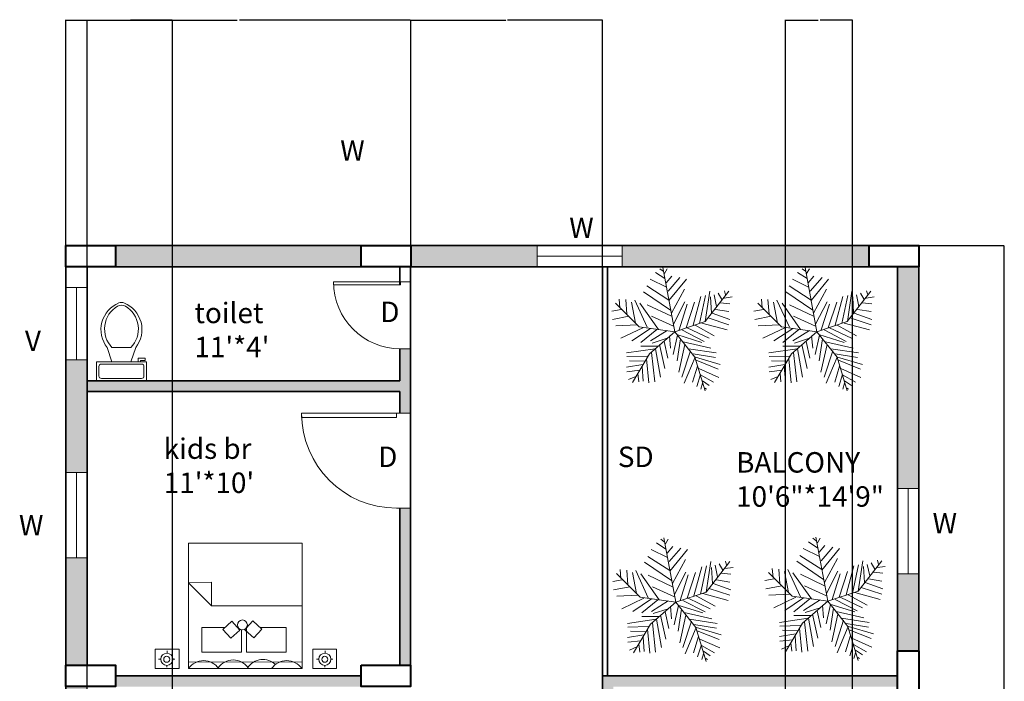
# Model space of a CAD drawing. Units: inches. Extents: x 1568 to 2529, y 2149 to 2897.
# Tile 16 of 16: x 2113 to 2529, y 2618 to 2897. Entities that reach past the tile are written whole.
import ezdxf

# ---------------------------------------------------------------- set-up
doc = ezdxf.new("R2010")
doc.units = ezdxf.units.IN
for name, color, linetype, lineweight in [('A-ANNO-DIMS', 2, 'Continuous', 18), ('A-AREA-IDEN', 210, 'Continuous', 18), ('A-COLS', 7, 'Continuous', 40), ('A-DOOR', 4, 'Continuous', 18), ('A-FLOR-FIXT', 9, 'Continuous', 18), ('A-FURN', 8, 'Continuous', 18), ('A-WALL-PATT', 172, 'Continuous', 13), ('text', 210, 'Continuous', 18), ('TREE', 94, 'Continuous', 13), ('wall', 7, 'Continuous', 35), ('window', 130, 'Continuous', 18)]:
    doc.layers.add(name, color=color, linetype=linetype, lineweight=lineweight)
doc.styles.get("Standard").update_dxf_attribs({"font": 'arial.ttf'})
doc.dimstyles.get("Standard").update_dxf_attribs({"dimtxt": 0.18, "dimasz": 0.18, "dimexe": 0.18, "dimexo": 0.0625, "dimgap": 0.09, "dimtad": 0, "dimtih": 1, "dimtoh": 1, "dimdec": 4, "dimzin": 0, "dimdsep": 46, "dimtxsty": 'Standard', "dimcen": 0.09, "dimadec": 0, "dimazin": 0, "dimtfac": 1, "dimtdec": 4, "dimtofl": 0, "dimtmove": 0, "dimatfit": 3, "dimfxl": 1, "dimtolj": 1, "dimtzin": 0, "dimarcsym": 0})

# ---------------------------------------------------------------- blocks, each defined once
blk = doc.blocks.new('*U4')
for p, q in [((9.5, -6), (9.5, -2)), ((-8, -8.5), (-8, -8)), ((-7, -8), (-7, -9.5)), ((-4, -8), (-6, -14)), ((4, -8), (6, -14)), ((-10, -8.5), (-8, -8.5)), ((-10, -9.5), (-10, -8.5)), ((-7, -9.5), (-10, -9.5)), ((4, -14), (-4, -14))]:
    blk.add_line(p, q)
blk.add_lwpolyline([(10.5, -8), (10.5, 0), (-10.5, 0), (-10.5, -8)], close=True)
for points in [[(-9.5, -2), (-9.5, -6)], [(8.5, -1), (-8.5, -1)], [(-8.5, -7), (8.5, -7)]]:
    blk.add_lwpolyline(points)
for centre, radius, start, end in [((-8.62, -1.88), 0.884, 81.8699, 188.1301), ((8.62, -1.88), 0.884, 351.8699, 98.1301), ((-8.62, -6.12), 0.884, 171.8699, 278.1301), ((8.62, -6.12), 0.884, 261.8699, 8.1301), ((3.52, -21.58), 12.17, 141.4691, 247.9714), ((4.2, -21.82), 11.33, 136.3677, 238.9468), ((-3.52, -21.58), 12.17, 292.0284, 38.5307), ((-4.2, -21.82), 11.33, 301.053, 43.6321), ((0, -27.88), 4, 245.7318, 294.2682), ((0, -29), 4, 254.8605, 285.1395)]:
    blk.add_arc(centre, radius, start, end)
blk = doc.blocks.new('*U2')
for p, q in [((0, 0), (0, -6)), ((40, 0), (40, -6))]:
    blk.add_line(p, q)
blk.add_lwpolyline([(0, 0), (0, 40), (1.75, 40), (1.75, 0)], close=True)
blk.add_arc((0, 0), 40, 0, 90)
blk = doc.blocks.new('*U10')
for p, q in [((-8.737, 47.138), (-17.069, 52.711)), ((-10.186, 53.64), (-13.084, 55.962)), ((0, 0), (-10.5, 57)), ((-9.099, 51.782), (-6.563, 55.962)), ((-7.288, 39.707), (-21.778, 46.673)), ((-7.65, 43.423), (-2.578, 49.46)), ((-5.839, 35.992), (4.667, 48.067)), ((-5.114, 27.632), (10.463, 46.673)), ((-3.665, 19.273), (-27.574, 35.527)), ((-5.114, 28.097), (-24.676, 40.636)), ((-2.941, 16.486), (8.652, 37.85)), ((27, 9), (48, 36)), ((27.127, 9.056), (31.112, 35.992)), ((44.153, 36.456), (45.239, 32.741)), ((-48.585, 21.131), (-49.309, 29.026)), ((-43.513, 28.561), (-42.427, 15.558)), ((-38.442, 26.239), (-34.819, 7.663)), ((-35.544, 28.097), (-24.314, 3.947)), ((-1.129, 6.734), (9.014, 26.704)), ((10.101, 3.483), (17.708, 26.239)), ((16.259, 5.805), (23.142, 31.348)), ((22.055, 7.198), (27.489, 32.277)), ((31.836, 30.883), (32.561, 16.486)), ((35.096, 32.741), (37.27, 22.524)), ((38.719, 34.134), (41.979, 28.561)), ((43.791, 29.954), (51.036, 30.883)), ((-47.498, 19.737), (-55.83, 18.344)), ((-31.5, 4.5), (-52.5, 25.5)), ((-14.533, 2.09), (-30.834, 25.31)), ((-24.314, 23.917), (-2.941, 13.7)), ((3.942, 1.625), (11.187, 24.381)), ((36.183, 19.737), (48.137, 17.88)), ((40.53, 25.775), (48.862, 24.846)), ((-40.615, 13.7), (-55.105, 10.913)), ((-20.691, 13.7), (-1.129, 4.876)), ((0, 0), (27, 9)), ((29.662, 12.307), (48.137, 6.269)), ((33.285, 16.486), (48.862, 10.913)), ((-33.37, 6.269), (-52.207, 5.34)), ((-28.299, 3.483), (-47.86, -5.805)), ((-21.416, 3.018), (-38.079, -8.128)), ((0, 0), (-31.5, 4.5)), ((-15.982, 2.09), (-30.11, -9.521)), ((0, 0), (-22.5, -19.5)), ((-6.563, 1.161), (-21.416, -8.128)), ((0, 0), (18, -22.5)), ((6.478, 1.625), (26.04, -8.592)), ((11.187, 3.483), (30.749, -5.805)), ((18.07, 5.805), (35.096, -3.483)), ((24.229, 7.663), (46.688, 1.625)), ((-6.563, -5.805), (-19.967, -9.985)), ((-9.461, -8.592), (-6.201, -23.453)), ((-4.752, -3.483), (-3.665, -14.629)), ((2.493, -3.019), (-1.491, -20.202)), ((1.769, -2.555), (24.229, -9.521)), ((5.029, -6.27), (2.131, -25.775)), ((-17.431, -15.094), (-42.789, -18.809)), ((-15.257, -12.772), (-30.11, -12.772)), ((-17.069, -15.094), (-12.721, -40.172)), ((-13.446, -11.378), (-8.737, -32.741)), ((9.014, -11.378), (3.58, -35.992)), ((14.085, -16.951), (6.478, -40.172)), ((7.565, -9.056), (32.198, -14.629)), ((12.274, -15.094), (36.907, -18.809)), ((-24.314, -21.596), (-42.427, -22.06)), ((-26.849, -26.24), (-40.253, -25.775)), ((-22.5, -19.5), (-37.5, -45)), ((-25.038, -23.918), (-22.865, -45.281)), ((-20.691, -18.345), (-17.793, -44.352)), ((18.07, -22.524), (8.289, -45.745)), ((16.259, -19.738), (36.183, -22.989)), ((18, -22.5), (27, -52.5)), ((18.433, -22.524), (40.53, -29.026)), ((19.157, -25.311), (38.719, -33.206)), ((-28.299, -29.026), (-42.789, -31.348)), ((-30.834, -34.135), (-42.427, -35.528)), ((-29.023, -30.884), (-27.936, -43.887)), ((20.244, -30.419), (15.897, -44.816)), ((21.331, -32.741), (39.081, -40.636)), ((-34.457, -39.708), (-40.978, -42.494)), ((-32.646, -36.921), (-31.921, -44.352)), ((22.78, -37.85), (19.519, -48.532)), ((22.78, -38.314), (34.372, -44.816)), ((24.591, -43.423), (30.749, -47.603)), ((24.591, -45.745), (23.142, -50.854)), ((26.764, -49.925), (28.213, -50.854))]:
    blk.add_line(p, q)
blk = doc.blocks.new('BED-WITH-NIGHTSTANDS')
for p, q in [((14.05, 36.12), (23.68, 36.4)), ((23.68, 26.45), (14.05, 36.12)), ((23.68, 36.4), (23.68, 26.45)), ((61.95, 26.45), (23.68, 26.45)), ((38.35, 16.98), (38.35, 15.84)), ((38.01, 16.14), (37.63, 16.49)), ((38.35, 15.84), (38.01, 16.14)), ((5, 6.48), (5, 7.42)), ((71.71, 6.48), (71.71, 7.42)), ((2.29, 3.95), (1.38, 3.95)), ((4.92, 1.35), (4.92, 0.55)), ((7.42, 3.92), (8.29, 3.92)), ((14.05, 2.79), (61.95, 2.73)), ((69, 3.95), (68.1, 3.95)), ((71.64, 1.35), (71.64, 0.55)), ((74.13, 3.92), (75, 3.92))]:
    blk.add_line(p, q)
for points in [[(14.05, 0), (61.95, 0), (61.95, 52.9), (14.05, 52.9)], [(31.9, 12.77), (35.7, 16.21), (32.32, 19.94), (28.52, 16.5)], [(10.04, 0), (0, 0), (0, 8.21), (10.04, 8.21)], [(76.49, 0), (66.44, 0), (66.44, 8.21), (76.49, 8.21)]]:
    blk.add_lwpolyline(points, close=True)
for points in [[(29.36, 17.26), (19.65, 17.26), (19.65, 6.93), (36.45, 6.93), (36.45, 16.34)], [(35.04, 17.26), (34.75, 17.26)], [(38.35, 16.98), (41.16, 20.08), (44.96, 16.64), (41.58, 12.91), (38.01, 16.14)], [(38.52, 17.23), (38.52, 6.93), (55.32, 6.93), (55.32, 17.26), (44.28, 17.26)], [(38.6, 17.26), (38.54, 17.26)]]:
    blk.add_lwpolyline(points)
for centre, radius in [((36.79, 18.4), 2.09), ((4.85, 3.92), 2.56), ((4.85, 3.92), 1.27), ((71.57, 3.92), 2.56), ((71.57, 3.92), 1.27)]:
    blk.add_circle(centre, radius)
for centre, start in [((20.4, -4.37), 34.5304), ((32.9, -4.09), 34.5304), ((45.42, -3.86), 46.3255), ((55.47, -4.37), 34.5304)]:
    blk.add_arc(centre, 7.71, start, 145.4696)
blk = doc.blocks.new('*D38')
at = {"layer": 'A-ANNO-DIMS', "color": 0, "lineweight": -2, "transparency": 16777216}
for p, q in [((2492.94, 2801.53), (2528.91, 2801.53)), ((2528.73, 2801.35), (2528.73, 2501.71)), ((2528.73, 2201.71), (2528.73, 2501.35)), ((2492.91, 2201.53), (2528.91, 2201.53))]:
    blk.add_line(p, q, dxfattribs=at)
at = {"layer": 'A-ANNO-DIMS', "color": 0, "transparency": 16777216}
for points in [[(2528.7, 2801.35), (2528.76, 2801.35), (2528.73, 2801.53)], [(2528.7, 2201.71), (2528.76, 2201.71), (2528.73, 2201.53)]]:
    blk.add_solid(points, dxfattribs=at)
at = {"layer": 'Defpoints', "color": 0, "transparency": 16777216}
for p in [(2492.88, 2801.53), (2528.73, 2801.53), (2492.85, 2201.53)]:
    blk.add_point(p, dxfattribs=at)
at = {"layer": 'A-ANNO-DIMS', "color": 0, "transparency": 16777216, "insert": (2528.73, 2501.53), "char_height": 0.18, "attachment_point": 5}
blk.add_mtext('\\A1;600', dxfattribs=at)
blk = doc.blocks.new('*D42')
at = {"layer": 'A-ANNO-DIMS', "color": 0, "lineweight": -2, "transparency": 16777216}
for p, q in [((2141.85, 2579.59), (2141.85, 2896.84)), ((2142.03, 2896.66), (2159.63, 2896.66)), ((2177.67, 2896.66), (2160.07, 2896.66)), ((2177.85, 2579.59), (2177.85, 2896.84))]:
    blk.add_line(p, q, dxfattribs=at)
at = {"layer": 'A-ANNO-DIMS', "color": 0, "transparency": 16777216}
for points in [[(2142.03, 2896.69), (2142.03, 2896.63), (2141.85, 2896.66)], [(2177.67, 2896.69), (2177.67, 2896.63), (2177.85, 2896.66)]]:
    blk.add_solid(points, dxfattribs=at)
at = {"layer": 'Defpoints', "color": 0, "transparency": 16777216}
for p in [(2177.85, 2896.66), (2141.85, 2579.53), (2177.85, 2579.53)]:
    blk.add_point(p, dxfattribs=at)
at = {"layer": 'A-ANNO-DIMS', "color": 0, "transparency": 16777216, "insert": (2159.85, 2896.66), "char_height": 0.18, "attachment_point": 5}
blk.add_mtext('\\A1;36', dxfattribs=at)
blk = doc.blocks.new('*D43')
at = {"layer": 'A-ANNO-DIMS', "color": 0, "lineweight": -2, "transparency": 16777216}
for p, q in [((2132.85, 2801.59), (2132.85, 2896.84)), ((2133.03, 2896.66), (2205.17, 2896.66)), ((2278.21, 2896.66), (2206.08, 2896.66)), ((2278.39, 2801.59), (2278.39, 2896.84))]:
    blk.add_line(p, q, dxfattribs=at)
at = {"layer": 'A-ANNO-DIMS', "color": 0, "transparency": 16777216}
for points in [[(2133.03, 2896.69), (2133.03, 2896.63), (2132.85, 2896.66)], [(2278.21, 2896.69), (2278.21, 2896.63), (2278.39, 2896.66)]]:
    blk.add_solid(points, dxfattribs=at)
at = {"layer": 'Defpoints', "color": 0, "transparency": 16777216}
for p in [(2278.39, 2896.66), (2132.85, 2801.53), (2278.39, 2801.53)]:
    blk.add_point(p, dxfattribs=at)
at = {"layer": 'A-ANNO-DIMS', "color": 0, "transparency": 16777216, "insert": (2205.62, 2896.66), "char_height": 0.18, "attachment_point": 5}
blk.add_mtext('\\A1;145.54', dxfattribs=at)
blk = doc.blocks.new('*D44')
at = {"layer": 'A-ANNO-DIMS', "color": 0, "lineweight": -2, "transparency": 16777216}
for p, q in [((2278.39, 2801.59), (2278.39, 2896.84)), ((2278.57, 2896.66), (2318.48, 2896.66)), ((2359.17, 2896.66), (2319.27, 2896.66)), ((2359.35, 2792.59), (2359.35, 2896.84))]:
    blk.add_line(p, q, dxfattribs=at)
at = {"layer": 'A-ANNO-DIMS', "color": 0, "transparency": 16777216}
for points in [[(2278.57, 2896.69), (2278.57, 2896.63), (2278.39, 2896.66)], [(2359.17, 2896.69), (2359.17, 2896.63), (2359.35, 2896.66)]]:
    blk.add_solid(points, dxfattribs=at)
at = {"layer": 'Defpoints', "color": 0, "transparency": 16777216}
for p in [(2359.35, 2896.66), (2278.39, 2801.53), (2359.35, 2792.53)]:
    blk.add_point(p, dxfattribs=at)
at = {"layer": 'A-ANNO-DIMS', "color": 0, "transparency": 16777216, "insert": (2318.87, 2896.66), "char_height": 0.18, "attachment_point": 5}
blk.add_mtext('\\A1;80.96', dxfattribs=at)
blk = doc.blocks.new('*D45')
at = {"layer": 'A-ANNO-DIMS', "color": 0, "lineweight": -2, "transparency": 16777216}
for p, q in [((2436.62, 2416.09), (2436.62, 2896.84)), ((2436.8, 2896.66), (2450.31, 2896.66)), ((2464.75, 2896.66), (2451.24, 2896.66)), ((2464.93, 2416.09), (2464.93, 2896.84))]:
    blk.add_line(p, q, dxfattribs=at)
at = {"layer": 'A-ANNO-DIMS', "color": 0, "transparency": 16777216}
for points in [[(2436.8, 2896.69), (2436.8, 2896.63), (2436.62, 2896.66)], [(2464.75, 2896.69), (2464.75, 2896.63), (2464.93, 2896.66)]]:
    blk.add_solid(points, dxfattribs=at)
at = {"layer": 'Defpoints', "color": 0, "transparency": 16777216}
for p in [(2464.93, 2896.66), (2436.62, 2416.03), (2464.93, 2416.03)]:
    blk.add_point(p, dxfattribs=at)
at = {"layer": 'A-ANNO-DIMS', "color": 0, "transparency": 16777216, "insert": (2450.77, 2896.66), "char_height": 0.18, "attachment_point": 5}
blk.add_mtext('\\A1;28.305', dxfattribs=at)

msp = doc.modelspace()

# ---------------------------------------------------------------- hatches: boundary and pattern name
at = {"layer": 'A-WALL-PATT'}
h = msp.add_hatch(color=256, dxfattribs=at)
h.dxf.hatch_style = 1
h.paths.add_polyline_path([(2257.4593, 2801.532), (2153.7841, 2801.532), (2153.7841, 2792.532), (2257.4593, 2792.532)])
h.paths.add_polyline_path([(2331.7115, 2801.532), (2278.3925, 2801.532), (2278.3925, 2792.532), (2331.7115, 2792.532)])
h.paths.add_polyline_path([(2141.8509, 2753.3576), (2141.6865, 2753.3576), (2132.8509, 2753.3576), (2132.8509, 2705.9172), (2141.8509, 2705.9172)])
h.paths.add_polyline_path([(2278.3509, 2757.9833), (2274.1052, 2757.9833, -0.00224577), (2273.8509, 2757.9844), (2273.8509, 2744.532), (2141.8509, 2744.532), (2141.8509, 2740.032), (2273.8509, 2740.032), (2273.8509, 2730.8156), (2278.3509, 2730.8156), (2278.3509, 2740.032)])
h.paths.add_polyline_path([(2471.947, 2801.532), (2367.7115, 2801.532), (2367.7115, 2792.532), (2471.947, 2792.532)])
h.paths.add_polyline_path([(2402.7886, 2351.2573), (2436.5067, 2351.2573), (2436.5067, 2383.453), (2402.7886, 2383.453)], flags=9)
h.paths.add_polyline_path([(2363.115, 2703.2844), (2384.1733, 2703.2844), (2384.1733, 2721.0645), (2363.115, 2721.0645)], flags=9)
h.paths.add_polyline_path([(2367.7631, 2584.032), (2380.7818, 2584.032), (2380.7818, 2601.8121), (2367.7631, 2601.8121)], flags=9)
h.paths.add_polyline_path([(2412.2706, 2522.1491), (2473.8683, 2522.1491), (2473.8683, 2568.725), (2412.2706, 2568.725)], flags=9)
h.paths.add_polyline_path([(2412.2706, 2686.5293), (2474.6569, 2686.5293), (2474.6569, 2718.725), (2412.2706, 2718.725)], flags=9)
h.paths.add_polyline_path([(2305.8704, 2205.7429), (2329.6007, 2205.7429), (2329.6007, 2223.523), (2305.8704, 2223.523)], flags=9)
h.paths.add_polyline_path([(2312.4696, 2308.5242), (2328.1604, 2308.5242), (2328.1604, 2326.3043), (2312.4696, 2326.3043)], flags=9)
h.paths.add_polyline_path([(2253.7912, 2420.5203), (2266.8099, 2420.5203), (2266.8099, 2438.3004), (2253.7912, 2438.3004)], flags=9)
h.paths.add_polyline_path([(2261.5714, 2703.4315), (2274.5902, 2703.4315), (2274.5902, 2721.2116), (2261.5714, 2721.2116)], flags=9)
h.paths.add_polyline_path([(2277.898, 2569.2764), (2333.9221, 2569.2764), (2333.9221, 2601.4721), (2277.898, 2601.4721)], flags=9)
h.paths.add_polyline_path([(2176.0749, 2419.8331), (2231.9754, 2419.8331), (2231.9754, 2452.0288), (2176.0749, 2452.0288)], flags=9)
h.paths.add_polyline_path([(2213.9423, 2525.7697), (2252.2216, 2525.7697), (2252.2216, 2557.9653), (2213.9423, 2557.9653)], flags=9)
h.paths.add_polyline_path([(2170.6878, 2692.4783), (2211.1801, 2692.4783), (2211.1801, 2724.6739), (2170.6878, 2724.6739)], flags=9)
h.paths.add_polyline_path([(2262.4629, 2764.5694), (2275.4816, 2764.5694), (2275.4816, 2782.3495), (2262.4629, 2782.3495)], flags=9)
h.paths.add_polyline_path([(2183.6493, 2749.7187), (2217.3673, 2749.7187), (2217.3673, 2781.9143), (2183.6493, 2781.9143)], flags=9)
h = msp.add_hatch(color=256, dxfattribs=at)
h.dxf.hatch_style = 1
h.paths.add_polyline_path([(2492.8509, 2792.532), (2483.8509, 2792.532), (2483.8509, 2699.1671), (2492.8509, 2699.1671)])
h.paths.add_polyline_path([(2278.3509, 2690.8156), (2273.8509, 2690.8156), (2273.8509, 2624.532), (2278.3509, 2624.532)])
h.paths.add_polyline_path([(2257.4177, 2620.032), (2153.7841, 2620.032), (2153.7841, 2615.532), (2257.4177, 2615.532)])
h.paths.add_polyline_path([(2141.8509, 2669.9172), (2132.8509, 2669.9172), (2132.8509, 2624.532), (2141.8509, 2624.532)])
h.paths.add_polyline_path([(2402.7886, 2351.2573), (2436.5067, 2351.2573), (2436.5067, 2383.453), (2402.7886, 2383.453)], flags=9)
h.paths.add_polyline_path([(2363.115, 2703.2844), (2384.1733, 2703.2844), (2384.1733, 2721.0645), (2363.115, 2721.0645)], flags=9)
h.paths.add_polyline_path([(2367.7631, 2584.032), (2380.7818, 2584.032), (2380.7818, 2601.8121), (2367.7631, 2601.8121)], flags=9)
h.paths.add_polyline_path([(2412.2706, 2522.1491), (2473.8683, 2522.1491), (2473.8683, 2568.725), (2412.2706, 2568.725)], flags=9)
h.paths.add_polyline_path([(2412.2706, 2686.5293), (2474.6569, 2686.5293), (2474.6569, 2718.725), (2412.2706, 2718.725)], flags=9)
h.paths.add_polyline_path([(2305.8704, 2205.7429), (2329.6007, 2205.7429), (2329.6007, 2223.523), (2305.8704, 2223.523)], flags=9)
h.paths.add_polyline_path([(2312.4696, 2308.5242), (2328.1604, 2308.5242), (2328.1604, 2326.3043), (2312.4696, 2326.3043)], flags=9)
h.paths.add_polyline_path([(2253.7912, 2420.5203), (2266.8099, 2420.5203), (2266.8099, 2438.3004), (2253.7912, 2438.3004)], flags=9)
h.paths.add_polyline_path([(2261.5714, 2703.4315), (2274.5902, 2703.4315), (2274.5902, 2721.2116), (2261.5714, 2721.2116)], flags=9)
h.paths.add_polyline_path([(2262.4629, 2764.5694), (2275.4816, 2764.5694), (2275.4816, 2782.3495), (2262.4629, 2782.3495)], flags=9)
h.paths.add_polyline_path([(2277.898, 2569.2764), (2333.9221, 2569.2764), (2333.9221, 2601.4721), (2277.898, 2601.4721)], flags=9)
h.paths.add_polyline_path([(2176.0749, 2419.8331), (2231.9754, 2419.8331), (2231.9754, 2452.0288), (2176.0749, 2452.0288)], flags=9)
h.paths.add_polyline_path([(2213.9423, 2525.7697), (2252.2216, 2525.7697), (2252.2216, 2557.9653), (2213.9423, 2557.9653)], flags=9)
h.paths.add_polyline_path([(2170.6878, 2692.4783), (2211.1801, 2692.4783), (2211.1801, 2724.6739), (2170.6878, 2724.6739)], flags=9)
h.paths.add_polyline_path([(2183.6493, 2749.7187), (2217.3673, 2749.7187), (2217.3673, 2781.9143), (2183.6493, 2781.9143)], flags=9)
h = msp.add_hatch(color=256, dxfattribs=at)
h.dxf.hatch_style = 1
h.paths.add_polyline_path([(2141.8509, 2615.532), (2132.8509, 2615.532), (2132.8509, 2564.2764), (2141.8509, 2564.2764)])
h.paths.add_polyline_path([(2141.8509, 2528.2764), (2132.8509, 2528.2764), (2132.8509, 2436.512), (2141.8509, 2436.512), (2141.8509, 2459.532)])
h.paths.add_polyline_path([(2278.3509, 2464.032), (2253.6925, 2464.032), (2141.8509, 2464.032), (2141.8509, 2459.532), (2255.8509, 2459.532), (2273.8509, 2459.532), (2273.8509, 2451.2271), (2278.3509, 2451.2271)])
h.paths.add_polyline_path([(2141.8509, 2400.512), (2132.8509, 2400.512), (2132.8509, 2339.532), (2141.8509, 2339.532)])
h.paths.add_polyline_path([(2258.2144, 2339.532), (2153.7841, 2339.532), (2153.7841, 2330.532), (2258.2144, 2330.532)])
h.paths.add_polyline_path([(2291.8353, 2339.532), (2279.1476, 2339.532), (2279.1476, 2330.532), (2291.8353, 2330.532)])
h.paths.add_polyline_path([(2402.7886, 2351.2573), (2436.5067, 2351.2573), (2436.5067, 2383.453), (2402.7886, 2383.453)], flags=9)
h.paths.add_polyline_path([(2363.115, 2703.2844), (2384.1733, 2703.2844), (2384.1733, 2721.0645), (2363.115, 2721.0645)], flags=9)
h.paths.add_polyline_path([(2367.7631, 2584.032), (2380.7818, 2584.032), (2380.7818, 2601.8121), (2367.7631, 2601.8121)], flags=9)
h.paths.add_polyline_path([(2412.2706, 2522.1491), (2473.8683, 2522.1491), (2473.8683, 2568.725), (2412.2706, 2568.725)], flags=9)
h.paths.add_polyline_path([(2412.2706, 2686.5293), (2474.6569, 2686.5293), (2474.6569, 2718.725), (2412.2706, 2718.725)], flags=9)
h.paths.add_polyline_path([(2305.8704, 2205.7429), (2329.6007, 2205.7429), (2329.6007, 2223.523), (2305.8704, 2223.523)], flags=9)
h.paths.add_polyline_path([(2312.4696, 2308.5242), (2328.1604, 2308.5242), (2328.1604, 2326.3043), (2312.4696, 2326.3043)], flags=9)
h.paths.add_polyline_path([(2261.5714, 2703.4315), (2274.5902, 2703.4315), (2274.5902, 2721.2116), (2261.5714, 2721.2116)], flags=9)
h.paths.add_polyline_path([(2262.4629, 2764.5694), (2275.4816, 2764.5694), (2275.4816, 2782.3495), (2262.4629, 2782.3495)], flags=9)
h.paths.add_polyline_path([(2277.898, 2569.2764), (2333.9221, 2569.2764), (2333.9221, 2601.4721), (2277.898, 2601.4721)], flags=9)
h.paths.add_polyline_path([(2213.9423, 2525.7697), (2252.2216, 2525.7697), (2252.2216, 2557.9653), (2213.9423, 2557.9653)], flags=9)
h.paths.add_polyline_path([(2170.6878, 2692.4783), (2211.1801, 2692.4783), (2211.1801, 2724.6739), (2170.6878, 2724.6739)], flags=9)
h.paths.add_polyline_path([(2183.6493, 2749.7187), (2217.3673, 2749.7187), (2217.3673, 2781.9143), (2183.6493, 2781.9143)], flags=9)
h = msp.add_hatch(color=256, dxfattribs=at)
h.dxf.hatch_style = 1
h.paths.add_polyline_path([(2492.8509, 2663.1671), (2483.8509, 2663.1671), (2483.8509, 2630.5978), (2492.8509, 2630.5978)])
h.paths.add_polyline_path([(2492.8509, 2609.6646), (2483.8509, 2609.6646), (2483.8509, 2572.3679), (2492.8509, 2572.3679)])
h.paths.add_polyline_path([(2492.8509, 2536.3679), (2483.8509, 2536.3679), (2483.8509, 2476.032), (2483.8509, 2458.371), (2492.8509, 2458.371)])
h.paths.add_polyline_path([(2483.8509, 2620.032), (2361.425, 2620.032), (2359.3509, 2620.032), (2359.3509, 2607.8035), (2363.8509, 2607.8035), (2363.8509, 2615.532), (2483.8509, 2615.532)])
h.paths.add_polyline_path([(2402.7886, 2351.2573), (2436.5067, 2351.2573), (2436.5067, 2383.453), (2402.7886, 2383.453)], flags=9)
h.paths.add_polyline_path([(2412.2706, 2522.1491), (2473.8683, 2522.1491), (2473.8683, 2568.725), (2412.2706, 2568.725)], flags=9)
h.paths.add_polyline_path([(2305.8704, 2205.7429), (2329.6007, 2205.7429), (2329.6007, 2223.523), (2305.8704, 2223.523)], flags=9)
h.paths.add_polyline_path([(2312.4696, 2308.5242), (2328.1604, 2308.5242), (2328.1604, 2326.3043), (2312.4696, 2326.3043)], flags=9)
h.paths.add_polyline_path([(2253.7912, 2420.5203), (2266.8099, 2420.5203), (2266.8099, 2438.3004), (2253.7912, 2438.3004)], flags=9)
h.paths.add_polyline_path([(2261.5714, 2703.4315), (2274.5902, 2703.4315), (2274.5902, 2721.2116), (2261.5714, 2721.2116)], flags=9)
h.paths.add_polyline_path([(2262.4629, 2764.5694), (2275.4816, 2764.5694), (2275.4816, 2782.3495), (2262.4629, 2782.3495)], flags=9)
h.paths.add_polyline_path([(2277.898, 2569.2764), (2333.9221, 2569.2764), (2333.9221, 2601.4721), (2277.898, 2601.4721)], flags=9)
h.paths.add_polyline_path([(2176.0749, 2419.8331), (2231.9754, 2419.8331), (2231.9754, 2452.0288), (2176.0749, 2452.0288)], flags=9)
h.paths.add_polyline_path([(2213.9423, 2525.7697), (2252.2216, 2525.7697), (2252.2216, 2557.9653), (2213.9423, 2557.9653)], flags=9)
h.paths.add_polyline_path([(2170.6878, 2692.4783), (2211.1801, 2692.4783), (2211.1801, 2724.6739), (2170.6878, 2724.6739)], flags=9)
h.paths.add_polyline_path([(2183.6493, 2749.7187), (2217.3673, 2749.7187), (2217.3673, 2781.9143), (2183.6493, 2781.9143)], flags=9)
h = msp.add_hatch(color=256, dxfattribs=at)
h.dxf.hatch_style = 1
h.paths.add_polyline_path([(2471.9177, 2339.532), (2463.2103, 2339.532), (2350.013, 2339.532), (2311.8757, 2339.532), (2291.8353, 2339.532), (2291.8353, 2335.032), (2313.7499, 2335.032), (2349.7476, 2335.032), (2349.7476, 2330.532), (2471.9177, 2330.532)])
h.paths.add_polyline_path([(2363.115, 2703.2844), (2384.1733, 2703.2844), (2384.1733, 2721.0645), (2363.115, 2721.0645)], flags=9)
h.paths.add_polyline_path([(2367.7631, 2584.032), (2380.7818, 2584.032), (2380.7818, 2601.8121), (2367.7631, 2601.8121)], flags=9)
h.paths.add_polyline_path([(2412.2706, 2522.1491), (2473.8683, 2522.1491), (2473.8683, 2568.725), (2412.2706, 2568.725)], flags=9)
h.paths.add_polyline_path([(2412.2706, 2686.5293), (2474.6569, 2686.5293), (2474.6569, 2718.725), (2412.2706, 2718.725)], flags=9)
h.paths.add_polyline_path([(2253.7912, 2420.5203), (2266.8099, 2420.5203), (2266.8099, 2438.3004), (2253.7912, 2438.3004)], flags=9)
h.paths.add_polyline_path([(2261.5714, 2703.4315), (2274.5902, 2703.4315), (2274.5902, 2721.2116), (2261.5714, 2721.2116)], flags=9)
h.paths.add_polyline_path([(2262.4629, 2764.5694), (2275.4816, 2764.5694), (2275.4816, 2782.3495), (2262.4629, 2782.3495)], flags=9)
h.paths.add_polyline_path([(2277.898, 2569.2764), (2333.9221, 2569.2764), (2333.9221, 2601.4721), (2277.898, 2601.4721)], flags=9)
h.paths.add_polyline_path([(2176.0749, 2419.8331), (2231.9754, 2419.8331), (2231.9754, 2452.0288), (2176.0749, 2452.0288)], flags=9)
h.paths.add_polyline_path([(2213.9423, 2525.7697), (2252.2216, 2525.7697), (2252.2216, 2557.9653), (2213.9423, 2557.9653)], flags=9)
h.paths.add_polyline_path([(2170.6878, 2692.4783), (2211.1801, 2692.4783), (2211.1801, 2724.6739), (2170.6878, 2724.6739)], flags=9)
h.paths.add_polyline_path([(2183.6493, 2749.7187), (2217.3673, 2749.7187), (2217.3673, 2781.9143), (2183.6493, 2781.9143)], flags=9)
h = msp.add_hatch(color=256, dxfattribs=at)
h.dxf.hatch_style = 1
h.paths.add_polyline_path([(2492.8509, 2422.371), (2483.8509, 2422.371), (2483.8509, 2339.532), (2492.8509, 2339.532)])
h.paths.add_polyline_path([(2483.8509, 2416.032), (2464.9258, 2416.032), (2464.9258, 2411.7863), (2464.9258, 2411.532), (2483.8509, 2411.532)])
h.paths.add_polyline_path([(2402.7886, 2351.2573), (2436.5067, 2351.2573), (2436.5067, 2383.453), (2402.7886, 2383.453)], flags=9)
h.paths.add_polyline_path([(2363.115, 2703.2844), (2384.1733, 2703.2844), (2384.1733, 2721.0645), (2363.115, 2721.0645)], flags=9)
h.paths.add_polyline_path([(2367.7631, 2584.032), (2380.7818, 2584.032), (2380.7818, 2601.8121), (2367.7631, 2601.8121)], flags=9)
h.paths.add_polyline_path([(2412.2706, 2522.1491), (2473.8683, 2522.1491), (2473.8683, 2568.725), (2412.2706, 2568.725)], flags=9)
h.paths.add_polyline_path([(2412.2706, 2686.5293), (2474.6569, 2686.5293), (2474.6569, 2718.725), (2412.2706, 2718.725)], flags=9)
h.paths.add_polyline_path([(2305.8704, 2205.7429), (2329.6007, 2205.7429), (2329.6007, 2223.523), (2305.8704, 2223.523)], flags=9)
h.paths.add_polyline_path([(2312.4696, 2308.5242), (2328.1604, 2308.5242), (2328.1604, 2326.3043), (2312.4696, 2326.3043)], flags=9)
h.paths.add_polyline_path([(2253.7912, 2420.5203), (2266.8099, 2420.5203), (2266.8099, 2438.3004), (2253.7912, 2438.3004)], flags=9)
h.paths.add_polyline_path([(2261.5714, 2703.4315), (2274.5902, 2703.4315), (2274.5902, 2721.2116), (2261.5714, 2721.2116)], flags=9)
h.paths.add_polyline_path([(2262.4629, 2764.5694), (2275.4816, 2764.5694), (2275.4816, 2782.3495), (2262.4629, 2782.3495)], flags=9)
h.paths.add_polyline_path([(2277.898, 2569.2764), (2333.9221, 2569.2764), (2333.9221, 2601.4721), (2277.898, 2601.4721)], flags=9)
h.paths.add_polyline_path([(2176.0749, 2419.8331), (2231.9754, 2419.8331), (2231.9754, 2452.0288), (2176.0749, 2452.0288)], flags=9)
h.paths.add_polyline_path([(2213.9423, 2525.7697), (2252.2216, 2525.7697), (2252.2216, 2557.9653), (2213.9423, 2557.9653)], flags=9)
h.paths.add_polyline_path([(2170.6878, 2692.4783), (2211.1801, 2692.4783), (2211.1801, 2724.6739), (2170.6878, 2724.6739)], flags=9)
h.paths.add_polyline_path([(2183.6493, 2749.7187), (2217.3673, 2749.7187), (2217.3673, 2781.9143), (2183.6493, 2781.9143)], flags=9)
h = msp.add_hatch(color=256, dxfattribs=at)
h.dxf.hatch_style = 1
h.paths.add_polyline_path([(2436.6209, 2416.032), (2363.8509, 2416.032), (2363.8509, 2411.532), (2436.6209, 2411.532)])
h.paths.add_polyline_path([(2363.115, 2703.2844), (2384.1733, 2703.2844), (2384.1733, 2721.0645), (2363.115, 2721.0645)], flags=9)
h.paths.add_polyline_path([(2367.7631, 2584.032), (2380.7818, 2584.032), (2380.7818, 2601.8121), (2367.7631, 2601.8121)], flags=9)
h.paths.add_polyline_path([(2412.2706, 2522.1491), (2473.8683, 2522.1491), (2473.8683, 2568.725), (2412.2706, 2568.725)], flags=9)
h.paths.add_polyline_path([(2412.2706, 2686.5293), (2474.6569, 2686.5293), (2474.6569, 2718.725), (2412.2706, 2718.725)], flags=9)
h.paths.add_polyline_path([(2261.5714, 2703.4315), (2274.5902, 2703.4315), (2274.5902, 2721.2116), (2261.5714, 2721.2116)], flags=9)
h.paths.add_polyline_path([(2262.4629, 2764.5694), (2275.4816, 2764.5694), (2275.4816, 2782.3495), (2262.4629, 2782.3495)], flags=9)
h.paths.add_polyline_path([(2277.898, 2569.2764), (2333.9221, 2569.2764), (2333.9221, 2601.4721), (2277.898, 2601.4721)], flags=9)
h.paths.add_polyline_path([(2213.9423, 2525.7697), (2252.2216, 2525.7697), (2252.2216, 2557.9653), (2213.9423, 2557.9653)], flags=9)
h.paths.add_polyline_path([(2170.6878, 2692.4783), (2211.1801, 2692.4783), (2211.1801, 2724.6739), (2170.6878, 2724.6739)], flags=9)
h.paths.add_polyline_path([(2183.6493, 2749.7187), (2217.3673, 2749.7187), (2217.3673, 2781.9143), (2183.6493, 2781.9143)], flags=9)
h.paths.add_polyline_path([(2402.7886, 2351.2573), (2436.5067, 2351.2573), (2436.5067, 2383.453), (2402.7886, 2383.453)], flags=9)
h.paths.add_polyline_path([(2305.8704, 2205.7429), (2329.6007, 2205.7429), (2329.6007, 2223.523), (2305.8704, 2223.523)], flags=9)
h.paths.add_polyline_path([(2312.4696, 2308.5242), (2328.1604, 2308.5242), (2328.1604, 2326.3043), (2312.4696, 2326.3043)], flags=9)
h.paths.add_polyline_path([(2253.7912, 2420.5203), (2266.8099, 2420.5203), (2266.8099, 2438.3004), (2253.7912, 2438.3004)], flags=9)
h.paths.add_polyline_path([(2176.0749, 2419.8331), (2231.9754, 2419.8331), (2231.9754, 2452.0288), (2176.0749, 2452.0288)], flags=9)
h = msp.add_hatch(color=256, dxfattribs=at)
h.dxf.hatch_style = 1
h.paths.add_polyline_path([(2278.3509, 2411.2271), (2273.8509, 2411.2271), (2273.8509, 2339.532), (2278.3509, 2339.532)])
h.paths.add_polyline_path([(2363.115, 2703.2844), (2384.1733, 2703.2844), (2384.1733, 2721.0645), (2363.115, 2721.0645)], flags=9)
h.paths.add_polyline_path([(2367.7631, 2584.032), (2380.7818, 2584.032), (2380.7818, 2601.8121), (2367.7631, 2601.8121)], flags=9)
h.paths.add_polyline_path([(2412.2706, 2522.1491), (2473.8683, 2522.1491), (2473.8683, 2568.725), (2412.2706, 2568.725)], flags=9)
h.paths.add_polyline_path([(2412.2706, 2686.5293), (2474.6569, 2686.5293), (2474.6569, 2718.725), (2412.2706, 2718.725)], flags=9)
h.paths.add_polyline_path([(2261.5714, 2703.4315), (2274.5902, 2703.4315), (2274.5902, 2721.2116), (2261.5714, 2721.2116)], flags=9)
h.paths.add_polyline_path([(2262.4629, 2764.5694), (2275.4816, 2764.5694), (2275.4816, 2782.3495), (2262.4629, 2782.3495)], flags=9)
h.paths.add_polyline_path([(2277.898, 2569.2764), (2333.9221, 2569.2764), (2333.9221, 2601.4721), (2277.898, 2601.4721)], flags=9)
h.paths.add_polyline_path([(2213.9423, 2525.7697), (2252.2216, 2525.7697), (2252.2216, 2557.9653), (2213.9423, 2557.9653)], flags=9)
h.paths.add_polyline_path([(2170.6878, 2692.4783), (2211.1801, 2692.4783), (2211.1801, 2724.6739), (2170.6878, 2724.6739)], flags=9)
h.paths.add_polyline_path([(2183.6493, 2749.7187), (2217.3673, 2749.7187), (2217.3673, 2781.9143), (2183.6493, 2781.9143)], flags=9)

# ---------------------------------------------------------------- linework, layer by layer
at = {"layer": 'A-COLS'}
for points in [[(2132.8509, 2801.532), (2153.7841, 2801.532), (2153.7841, 2792.532), (2132.8509, 2792.532)], [(2257.4593, 2801.532), (2278.3925, 2801.532), (2278.3925, 2792.532), (2257.4593, 2792.532)], [(2471.947, 2801.532), (2492.8802, 2801.532), (2492.8802, 2792.532), (2471.947, 2792.532)], [(2492.8509, 2630.5978), (2492.8509, 2609.6646), (2483.8509, 2609.6646), (2483.8509, 2630.5978)], [(2132.8509, 2624.532), (2153.7841, 2624.532), (2153.7841, 2615.532), (2132.8509, 2615.532)], [(2257.4177, 2624.532), (2278.3509, 2624.532), (2278.3509, 2615.532), (2257.4177, 2615.532)]]:
    msp.add_lwpolyline(points, close=True, dxfattribs=at)
at = {"layer": 'wall'}
for p, q in [((2141.8509, 2792.532), (2273.8509, 2792.532)), ((2273.8509, 2792.532), (2273.8509, 2785.0499)), ((2278.3509, 2792.532), (2278.3509, 2740.032)), ((2359.3509, 2600.532), (2359.3509, 2792.532)), ((2361.425, 2620.032), (2361.425, 2792.532)), ((2483.8509, 2792.532), (2423.8509, 2792.532)), ((2483.8509, 2792.532), (2483.8509, 2615.532)), ((2273.8509, 2757.9844), (2273.8509, 2744.532)), ((2273.8509, 2744.532), (2141.8509, 2744.532)), ((2273.8509, 2740.032), (2141.8509, 2740.032)), ((2273.8509, 2740.032), (2273.8509, 2730.8156)), ((2278.3509, 2740.032), (2278.3509, 2615.532)), ((2273.8509, 2690.8156), (2273.8509, 2624.532)), ((2257.4177, 2620.032), (2153.7841, 2620.032)), ((2361.425, 2620.032), (2359.3509, 2620.032)), ((2483.8509, 2620.032), (2361.425, 2620.032))]:
    msp.add_line(p, q, dxfattribs=at)
msp.add_lwpolyline([(2132.8509, 2201.532), (2492.8509, 2201.532), (2492.8509, 2801.532), (2132.8509, 2801.532)], close=True, dxfattribs=at)
msp.add_lwpolyline([(2483.8509, 2395.032), (2483.8509, 2792.532), (2141.8509, 2792.532), (2141.8509, 2624.532)], dxfattribs=at)
at = {"layer": 'window'}
for p, q in [((2331.7115, 2801.532), (2331.7115, 2792.532)), ((2367.7115, 2801.532), (2367.7115, 2792.532)), ((2331.7115, 2797.032), (2367.7115, 2797.032)), ((2132.8509, 2783.8872), (2141.8509, 2783.8872)), ((2137.3509, 2753.3576), (2137.3509, 2783.8872)), ((2132.8509, 2753.3576), (2141.7162, 2753.3576)), ((2141.6865, 2753.3576), (2141.8509, 2753.3576)), ((2132.8509, 2705.9172), (2141.8509, 2705.9172)), ((2137.3509, 2669.9172), (2137.3509, 2705.9172)), ((2483.8509, 2699.1671), (2492.8509, 2699.1671)), ((2488.3509, 2663.1671), (2488.3509, 2699.1671)), ((2132.8509, 2669.9172), (2141.8509, 2669.9172)), ((2483.8509, 2663.1671), (2492.8509, 2663.1671))]:
    msp.add_line(p, q, dxfattribs=at)

# ---------------------------------------------------------------- block references
at = {"layer": 'A-DOOR', "xscale": -0.7076230433786183, "yscale": 0.7076230433786183, "zscale": 0.7076230433786183, "rotation": 90}
msp.add_blockref('*U2', (2274.1052, 2786.2882), dxfattribs=at)
at = {"layer": 'A-DOOR', "xscale": -1, "rotation": 90}
msp.add_blockref('*U2', (2272.3509, 2730.8156), dxfattribs=at)
at = {"layer": 'A-FLOR-FIXT', "rotation": 180}
msp.add_blockref('*U4', (2156.3167, 2744.532), dxfattribs=at)
at = {"layer": 'A-FURN'}
msp.add_blockref('BED-WITH-NIGHTSTANDS', (2170.5771, 2623.146), dxfattribs=at)
at = {"layer": 'TREE', "xscale": 0.4751991687393962, "yscale": 0.4751991687393962, "zscale": 0.4751991687393962}
for p in [(2389.8173, 2765.2128), (2449.8173, 2765.2128), (2390.234, 2651.1387), (2454.4, 2651.555)]:
    msp.add_blockref('*U10', p, dxfattribs=at)

# ---------------------------------------------------------------- texts
at = {"layer": 'A-AREA-IDEN', "attachment_point": 1}
for s, insert, char_height in [("toilet\\P11'*4'", (2187.1188, 2777.4737), 8.62815), ("kids br\\P11'*10'", (2174.1573, 2720.2333), 8.62815), ('BALCONY\\P10\'6"*14\'9"', (2415.7401, 2714.4374), 8.628146)]:
    msp.add_mtext_dynamic_manual_height_columns(s, width=94.297369, gutter_width=43.1407, heights=[0], dxfattribs=dict(at, insert=insert, char_height=char_height))
at = {"layer": 'text', "attachment_point": 1}
for s, insert, char_height in [('W', (2248.6381, 2845.9913), 8.6281), ('W', (2345.3058, 2813.3764), 8.6281), ('D', (2265.5498, 2777.9089), 8.6281), ('V', (2115.5632, 2765.7085), 8.6281), ('D', (2264.6584, 2716.771), 8.6281), ('SD', (2365.8135, 2716.771), 8.62815), ('W', (2498.6496, 2688.787), 8.6281), ('W', (2113.0523, 2687.9345), 8.6281)]:
    msp.add_mtext_dynamic_manual_height_columns(s, width=94.297369, gutter_width=43.1407, heights=[23.0437], dxfattribs=dict(at, insert=insert, char_height=char_height))

# ---------------------------------------------------------------- dimensions: what is measured, and where the dimension line sits
at = {"layer": 'A-ANNO-DIMS'}
for base, p1, p2, override, picture, middle in [((2278.3925, 2896.6572), (2132.8509, 2801.532), (2278.3925, 2801.532), {"dimdec": 2, "dimlfac": 1, "dimrnd": 0, "dimzin": 0, "dimdsep": 46, "dimlunit": 2}, '*D43', (2205.6217, 2896.6572)), ((2177.8509, 2896.6572), (2141.8509, 2579.532), (2177.8509, 2579.532), {"dimdec": 0, "dimlfac": 1, "dimrnd": 0, "dimzin": 0, "dimdsep": 46, "dimlunit": 2}, '*D42', (2159.8509, 2896.6572)), ((2359.3509, 2896.6572), (2278.3925, 2801.532), (2359.3509, 2792.532), {"dimdec": 2, "dimlfac": 1, "dimrnd": 0, "dimzin": 0, "dimdsep": 46, "dimlunit": 2}, '*D44', (2318.8717, 2896.6572)), ((2464.9258, 2896.6572), (2436.6209, 2416.032), (2464.9258, 2416.032), {"dimdec": 3, "dimlfac": 1, "dimrnd": 0, "dimzin": 0, "dimdsep": 46, "dimlunit": 2}, '*D45', (2450.7733, 2896.6572))]:
    dim = msp.add_linear_dim(base=base, p1=p1, p2=p2, dimstyle='Standard', override=override, dxfattribs=at)
    dim.commit()
    dim.dimension.update_dxf_attribs({"geometry": picture, "text_midpoint": middle})
dim = msp.add_linear_dim(base=(2528.7302, 2801.532), p1=(2492.8509, 2201.532), p2=(2492.8802, 2801.532), angle=90, dimstyle='Standard', override={"dimdec": 0, "dimlfac": 1, "dimrnd": 0, "dimzin": 0, "dimdsep": 46, "dimlunit": 2}, dxfattribs=at)
dim.commit()
dim.dimension.update_dxf_attribs({"geometry": '*D38', "text_midpoint": (2528.7302, 2501.532)})

doc.saveas('drawing.dxf')
